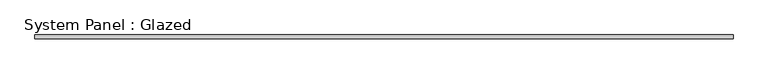
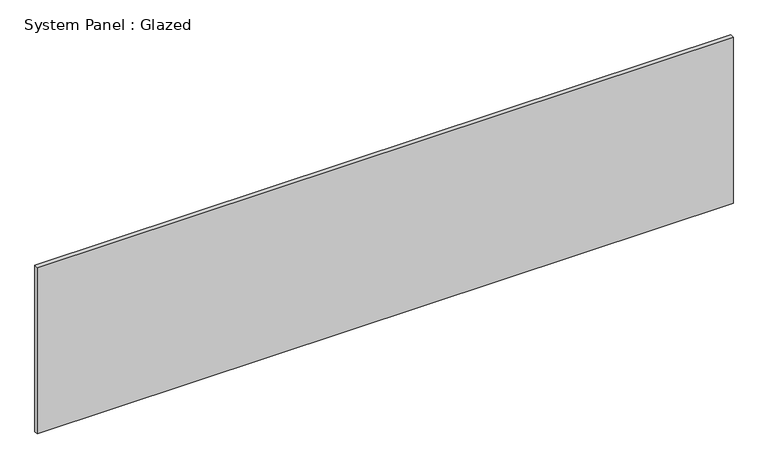
"""IFC4 building model written with IfcOpenShell, lengths in millimetres: plate geometry, System Panel : Glazed."""

from ifc_helpers import new_model, si_unit, origin, origin_with_axes, place, context, project, spatial, polyline, outline, extrude, source, transform, mapped, element, save


def system_panel_glazed_c0b1402d(model_context):
    return source(origin(), model_context, "Body", "SweptSolid", [
        extrude(outline(polyline([(2413.0, 19.05), (-2413.0, 19.05), (-2413.0, 44.45), (2413.0, 44.45), (2413.0, 19.05)])), origin_with_axes(), (0.0, 0.0, 1.0), 1219.2),
    ])


if __name__ == "__main__":
    model = new_model("IFC4")
    model_context = context("Model", 3, world=origin())
    ifc_project = project(units=[si_unit("LENGTHUNIT", "METRE", prefix="MILLI")], contexts=[model_context])
    site = spatial("IfcSite", under=ifc_project)
    building = spatial("IfcBuilding", under=site)
    placement = place(None, origin())
    system_panel_glazed_shape = system_panel_glazed_c0b1402d(model_context)
    element("IfcPlate", 1, ObjectType="System Panel : Glazed", at=placement, inside=building, context=model_context, shape_type="MappedRepresentation", body=[
        mapped(system_panel_glazed_shape, transform((0.0, 0.0, 0.0), x_axis=(1.0, 0.0, 0.0), y_axis=(0.0, 1.0, 0.0), z_axis=(0.0, 0.0, 1.0))),
    ])
    save(model, "model.ifc")

# Revit data of these elements
# Type "System Panel : Glazed"
#   Construction Type Id = "GSP4R"
#   Analytic Construction = "1/8 in Pilkington single glazing"
#   Visual Light Transmittance = 0.9
#   Solar Heat Gain Coefficient = 0.86
#   Heat Transfer Coefficient (U) = 1.18115 BTU/(h·ft²·°F)
# Element 1 (IfcPlate, "System Panel : Glazed")
#   Materials on its faces: "Glass"
# Materials
#   "Glass": class "Glass", colour RGB 0 128 192, transparency 0.75, Description = "Soda Lime Glass", Cost = 0
